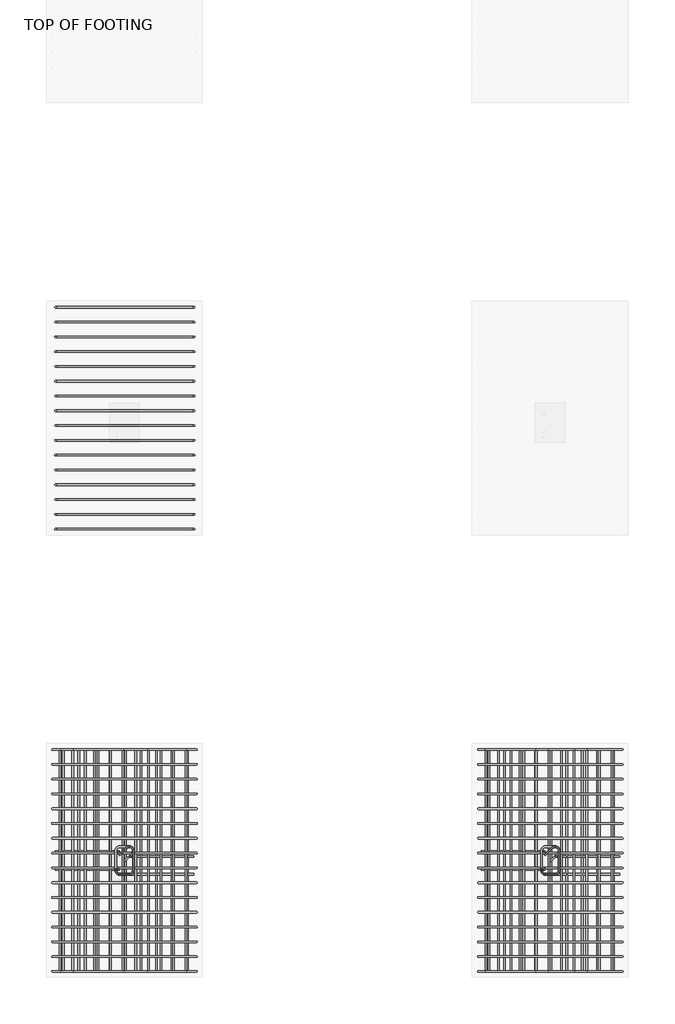
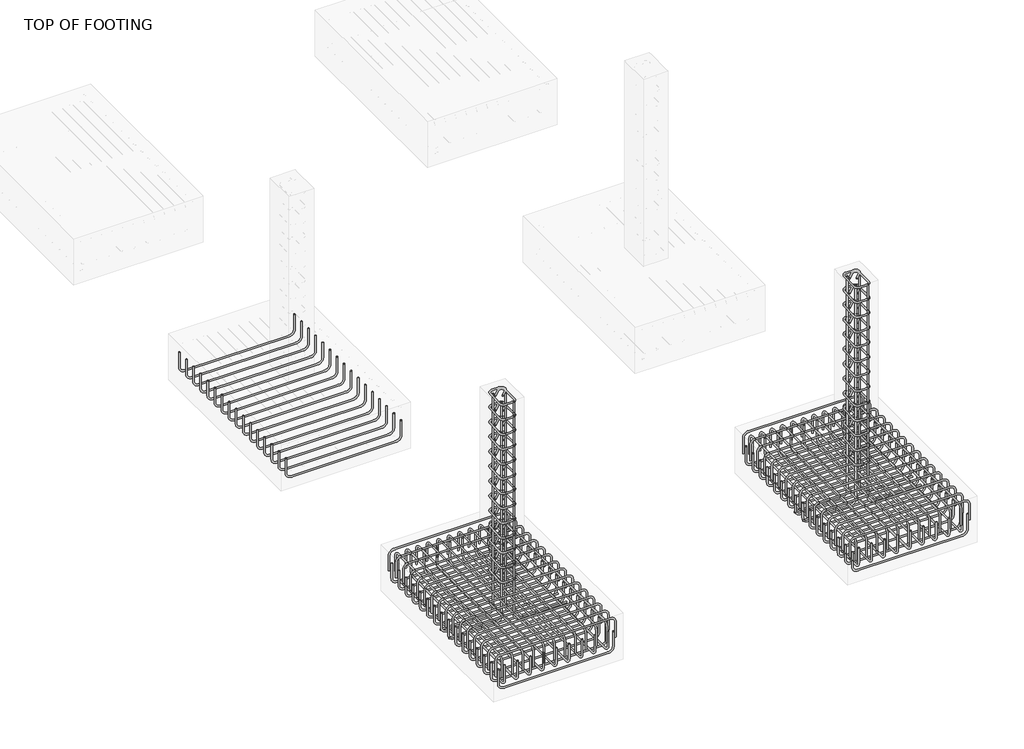
# One storey, part 2 of 8: 15 reinforcing bars.
"""IFC4 building model written with IfcOpenShell, lengths in millimetres."""

from ifc_helpers import new_model, si_unit, point, frame, origin, place, context, project, spatial, polyline, circle_curve, trimmed, segment, composite_curve, source, transform, mapped, element, save
from ifc_brep_helpers import swept_disk

model = new_model("IFC4")

# Units and contexts
model_context = context("Model", 3, world=origin())
ifc_project = project(units=[si_unit("LENGTHUNIT", "METRE", prefix="MILLI")], contexts=[model_context])

# Site, building, storey
site = spatial("IfcSite", under=ifc_project)
building = spatial("IfcBuilding", under=site)
storey = spatial("IfcBuildingStorey", under=building, Name="TOP OF FOOTING", Elevation=-1828.8)

# Reinforcing bars
placement = place(None, origin())
reinforcing_bar_shape = source(origin(), model_context, "Body", "SolidModel", [
    swept_disk(composite_curve([segment(polyline([(-4694.1573229, 6451.7662126, -2008.2544267), (-4694.1573229, 6451.7662126, -2155.5544267)]), True, "CONTINUOUS"), segment(trimmed(circle_curve(frame((-4740.5073229, 6451.7662126, -2155.5544267), z_axis=(0.0, 1.0, 0.0), x_axis=(46.350000000000364, 0.0, 0.0)), 46.35), [point((-4694.1573229, 6451.7662126, -2155.5544267))], [point((-4740.5073229, 6451.7662126, -2201.9044267))], True, "CARTESIAN"), True, "CONTINUOUS"), segment(polyline([(-4740.5073229, 6451.7662126, -2201.9044267), (-5711.5233592, 6451.7662126, -2201.9044267)]), True, "CONTINUOUS"), segment(trimmed(circle_curve(frame((-5711.5233592, 6451.7662126, -2155.5544267), z_axis=(0.0, 1.0, 0.0), x_axis=(0.0, 0.0, -46.34999999999991)), 46.35), [point((-5711.5233592, 6451.7662126, -2201.9044267))], [point((-5757.8733592, 6451.7662126, -2155.5544267))], True, "CARTESIAN"), True, "CONTINUOUS"), segment(polyline([(-5757.8733592, 6451.7662126, -2155.5544267), (-5757.8733592, 6451.7662126, -2008.2544267)]), True, "CONTINUOUS")], self_intersect=False), 6.35),
])
element("IfcReinforcingBar", 1, at=placement, inside=storey, context=model_context, shape_type="MappedRepresentation", body=[
    mapped(reinforcing_bar_shape, transform((0.0, 0.0, 0.0), x_axis=(1.0, 0.0, 0.0), y_axis=(0.0, 1.0, 0.0), z_axis=(0.0, 0.0, 1.0))),
    mapped(reinforcing_bar_shape, transform((0.0, -113.82, 0.0), x_axis=(1.0, 0.0, 0.0), y_axis=(0.0, 1.0, 0.0), z_axis=(0.0, 0.0, 1.0))),
    mapped(reinforcing_bar_shape, transform((0.0, -227.64, 0.0), x_axis=(1.0, 0.0, 0.0), y_axis=(0.0, 1.0, 0.0), z_axis=(0.0, 0.0, 1.0))),
    mapped(reinforcing_bar_shape, transform((0.0, -341.46, 0.0), x_axis=(1.0, 0.0, 0.0), y_axis=(0.0, 1.0, 0.0), z_axis=(0.0, 0.0, 1.0))),
    mapped(reinforcing_bar_shape, transform((0.0, -455.28, 0.0), x_axis=(1.0, 0.0, 0.0), y_axis=(0.0, 1.0, 0.0), z_axis=(0.0, 0.0, 1.0))),
    mapped(reinforcing_bar_shape, transform((0.0, -569.1, 0.0), x_axis=(1.0, 0.0, 0.0), y_axis=(0.0, 1.0, 0.0), z_axis=(0.0, 0.0, 1.0))),
    mapped(reinforcing_bar_shape, transform((0.0, -682.92, 0.0), x_axis=(1.0, 0.0, 0.0), y_axis=(0.0, 1.0, 0.0), z_axis=(0.0, 0.0, 1.0))),
    mapped(reinforcing_bar_shape, transform((0.0, -796.74, 0.0), x_axis=(1.0, 0.0, 0.0), y_axis=(0.0, 1.0, 0.0), z_axis=(0.0, 0.0, 1.0))),
    mapped(reinforcing_bar_shape, transform((0.0, -910.56, 0.0), x_axis=(1.0, 0.0, 0.0), y_axis=(0.0, 1.0, 0.0), z_axis=(0.0, 0.0, 1.0))),
    mapped(reinforcing_bar_shape, transform((0.0, -1024.38, 0.0), x_axis=(1.0, 0.0, 0.0), y_axis=(0.0, 1.0, 0.0), z_axis=(0.0, 0.0, 1.0))),
    mapped(reinforcing_bar_shape, transform((0.0, -1138.2, 0.0), x_axis=(1.0, 0.0, 0.0), y_axis=(0.0, 1.0, 0.0), z_axis=(0.0, 0.0, 1.0))),
    mapped(reinforcing_bar_shape, transform((0.0, -1252.02, 0.0), x_axis=(1.0, 0.0, 0.0), y_axis=(0.0, 1.0, 0.0), z_axis=(0.0, 0.0, 1.0))),
    mapped(reinforcing_bar_shape, transform((0.0, -1365.84, 0.0), x_axis=(1.0, 0.0, 0.0), y_axis=(0.0, 1.0, 0.0), z_axis=(0.0, 0.0, 1.0))),
    mapped(reinforcing_bar_shape, transform((0.0, -1479.66, 0.0), x_axis=(1.0, 0.0, 0.0), y_axis=(0.0, 1.0, 0.0), z_axis=(0.0, 0.0, 1.0))),
    mapped(reinforcing_bar_shape, transform((0.0, -1593.48, 0.0), x_axis=(1.0, 0.0, 0.0), y_axis=(0.0, 1.0, 0.0), z_axis=(0.0, 0.0, 1.0))),
    mapped(reinforcing_bar_shape, transform((0.0, -1707.3, 0.0), x_axis=(1.0, 0.0, 0.0), y_axis=(0.0, 1.0, 0.0), z_axis=(0.0, 0.0, 1.0))),
])
reinforcing_bar_2_shape = source(origin(), model_context, "Body", "SolidModel", [
    swept_disk(composite_curve([segment(polyline([(-5269.7182423, 2235.4007933, -46.35), (-5213.9746793, 2291.1443562, -46.35)]), True, "CONTINUOUS"), segment(trimmed(circle_curve(frame((-5191.8068817, 2268.9765586, -46.35), z_axis=(0.0, 0.0, -1.0), x_axis=(-22.167797600000085, 22.167797600000085, 0.0)), 31.35), [point((-5213.9746793, 2291.1443562, -46.35))], [point((-5160.4568817, 2268.9765586, -46.35))], True, "CARTESIAN"), True, "CONTINUOUS"), segment(polyline([(-5160.4568817, 2268.9765586, -46.35), (-5160.4568817, 2119.5765586, -46.35)]), True, "CONTINUOUS"), segment(trimmed(circle_curve(frame((-5191.8068817, 2119.5765586, -46.35), z_axis=(0.0, 0.0, -1.0), x_axis=(31.350000000000364, 0.0, 0.0)), 31.35), [point((-5160.4568817, 2119.5765586, -46.35))], [point((-5191.8068817, 2088.2265586, -46.35))], True, "CARTESIAN"), True, "CONTINUOUS"), segment(polyline([(-5191.8068817, 2088.2265586, -46.35), (-5265.0068817, 2088.2265586, -46.35)]), True, "CONTINUOUS"), segment(trimmed(circle_curve(frame((-5265.0068817, 2119.5205096, -44.4761991), z_axis=(0.0, 0.05977036468717588, -0.9982121535551258), x_axis=(0.0, -31.293951000000106, -1.873800899999999)), 31.35), [point((-5265.0068817, 2088.2265586, -46.35))], [point((-5296.3568817, 2119.5205096, -44.4761991))], True, "CARTESIAN"), True, "CONTINUOUS"), segment(polyline([(-5296.3568817, 2119.5205096, -44.4761991), (-5296.3568817, 2269.0326076, -35.5238009)]), True, "CONTINUOUS"), segment(trimmed(circle_curve(frame((-5265.0068817, 2269.0326076, -35.5238009), z_axis=(0.0, 0.05977036468717588, -0.9982121535551258), x_axis=(-31.349999999999454, 0.0, 0.0)), 31.35), [point((-5296.3568817, 2269.0326076, -35.5238009))], [point((-5265.0068817, 2300.3265586, -33.65))], True, "CARTESIAN"), True, "CONTINUOUS"), segment(polyline([(-5265.0068817, 2300.3265586, -33.65), (-5191.8068817, 2300.3265586, -33.65)]), True, "CONTINUOUS"), segment(trimmed(circle_curve(frame((-5191.8068817, 2268.9765586, -33.65), z_axis=(0.0, 0.0, -1.0), x_axis=(0.0, 31.350000000000364, 0.0)), 31.35), [point((-5191.8068817, 2300.3265586, -33.65))], [point((-5169.6390841, 2246.808761, -33.65))], True, "CARTESIAN"), True, "CONTINUOUS"), segment(polyline([(-5169.6390841, 2246.808761, -33.65), (-5225.3826471, 2191.0651981, -33.65)]), True, "CONTINUOUS")], self_intersect=False), 6.35),
])
element("IfcReinforcingBar", 2, at=placement, inside=storey, context=model_context, shape_type="MappedRepresentation", body=[
    mapped(reinforcing_bar_2_shape, transform((0.0, 0.0, 0.0), x_axis=(1.0, 0.0, 0.0), y_axis=(0.0, 1.0, 0.0), z_axis=(0.0, 0.0, 1.0))),
    mapped(reinforcing_bar_2_shape, transform((0.0, 0.0, -144.675), x_axis=(1.0, 0.0, 0.0), y_axis=(0.0, 1.0, 0.0), z_axis=(0.0, 0.0, 1.0))),
    mapped(reinforcing_bar_2_shape, transform((0.0, 0.0, -289.35), x_axis=(1.0, 0.0, 0.0), y_axis=(0.0, 1.0, 0.0), z_axis=(0.0, 0.0, 1.0))),
    mapped(reinforcing_bar_2_shape, transform((0.0, 0.0, -434.025), x_axis=(1.0, 0.0, 0.0), y_axis=(0.0, 1.0, 0.0), z_axis=(0.0, 0.0, 1.0))),
    mapped(reinforcing_bar_2_shape, transform((0.0, 0.0, -578.7), x_axis=(1.0, 0.0, 0.0), y_axis=(0.0, 1.0, 0.0), z_axis=(0.0, 0.0, 1.0))),
    mapped(reinforcing_bar_2_shape, transform((0.0, 0.0, -723.375), x_axis=(1.0, 0.0, 0.0), y_axis=(0.0, 1.0, 0.0), z_axis=(0.0, 0.0, 1.0))),
    mapped(reinforcing_bar_2_shape, transform((0.0, 0.0, -868.05), x_axis=(1.0, 0.0, 0.0), y_axis=(0.0, 1.0, 0.0), z_axis=(0.0, 0.0, 1.0))),
    mapped(reinforcing_bar_2_shape, transform((0.0, 0.0, -1012.725), x_axis=(1.0, 0.0, 0.0), y_axis=(0.0, 1.0, 0.0), z_axis=(0.0, 0.0, 1.0))),
    mapped(reinforcing_bar_2_shape, transform((0.0, 0.0, -1157.4), x_axis=(1.0, 0.0, 0.0), y_axis=(0.0, 1.0, 0.0), z_axis=(0.0, 0.0, 1.0))),
    mapped(reinforcing_bar_2_shape, transform((0.0, 0.0, -1302.075), x_axis=(1.0, 0.0, 0.0), y_axis=(0.0, 1.0, 0.0), z_axis=(0.0, 0.0, 1.0))),
    mapped(reinforcing_bar_2_shape, transform((0.0, 0.0, -1446.75), x_axis=(1.0, 0.0, 0.0), y_axis=(0.0, 1.0, 0.0), z_axis=(0.0, 0.0, 1.0))),
    mapped(reinforcing_bar_2_shape, transform((0.0, 0.0, -1591.425), x_axis=(1.0, 0.0, 0.0), y_axis=(0.0, 1.0, 0.0), z_axis=(0.0, 0.0, 1.0))),
    mapped(reinforcing_bar_2_shape, transform((0.0, 0.0, -1736.1), x_axis=(1.0, 0.0, 0.0), y_axis=(0.0, 1.0, 0.0), z_axis=(0.0, 0.0, 1.0))),
])
reinforcing_bar_3_shape = source(origin(), model_context, "Body", "SolidModel", [
    swept_disk(composite_curve([segment(polyline([(-4695.380398, 2088.2265586, -2177.1384798), (-5136.5372203, 2088.2265586, -2177.1384798)]), True, "CONTINUOUS"), segment(trimmed(circle_curve(frame((-5136.5372203, 2088.2265586, -2130.7884798), z_axis=(0.0, 1.0, 0.0), x_axis=(0.0, 0.0, -46.34999999999991)), 46.35), [point((-5136.5372203, 2088.2265586, -2177.1384798))], [point((-5182.8872203, 2088.2265586, -2130.7884798))], True, "CARTESIAN"), True, "CONTINUOUS"), segment(polyline([(-5182.8872203, 2088.2265586, -2130.7884798), (-5182.8872203, 2088.2265586, -40.0)]), True, "CONTINUOUS")], self_intersect=False), 6.35),
])
element("IfcReinforcingBar", 3, at=placement, inside=storey, context=model_context, shape_type="MappedRepresentation", body=[
    mapped(reinforcing_bar_3_shape, transform((0.0, 0.0, 0.0), x_axis=(1.0, 0.0, 0.0), y_axis=(0.0, 1.0, 0.0), z_axis=(0.0, 0.0, 1.0))),
    mapped(reinforcing_bar_3_shape, transform((0.0, 135.9, 0.0), x_axis=(1.0, 0.0, 0.0), y_axis=(0.0, 1.0, 0.0), z_axis=(0.0, 0.0, 1.0))),
])
reinforcing_bar_4_shape = source(origin(), model_context, "Body", "SolidModel", [
    swept_disk(composite_curve([segment(polyline([(-5761.4333654, 2126.3265586, -2177.1384798), (-5320.2765432, 2126.3265586, -2177.1384798)]), True, "CONTINUOUS"), segment(trimmed(circle_curve(frame((-5320.2765432, 2126.3265586, -2130.7884798), z_axis=(0.0, -1.0, 0.0), x_axis=(0.0, 0.0, -46.34999999999991)), 46.35), [point((-5320.2765432, 2126.3265586, -2177.1384798))], [point((-5273.9265432, 2126.3265586, -2130.7884798))], True, "CARTESIAN"), True, "CONTINUOUS"), segment(polyline([(-5273.9265432, 2126.3265586, -2130.7884798), (-5273.9265432, 2126.3265586, -40.0)]), True, "CONTINUOUS")], self_intersect=False), 6.35),
])
element("IfcReinforcingBar", 4, at=placement, inside=storey, context=model_context, shape_type="MappedRepresentation", body=[
    mapped(reinforcing_bar_4_shape, transform((0.0, 0.0, 0.0), x_axis=(1.0, 0.0, 0.0), y_axis=(0.0, 1.0, 0.0), z_axis=(0.0, 0.0, 1.0))),
    mapped(reinforcing_bar_4_shape, transform((0.0, 135.9, 0.0), x_axis=(1.0, 0.0, 0.0), y_axis=(0.0, 1.0, 0.0), z_axis=(0.0, 0.0, 1.0))),
])
reinforcing_bar_5_shape = source(origin(), model_context, "Body", "SolidModel", [
    swept_disk(composite_curve([segment(polyline([(-1993.1182423, 2235.4007933, -46.35), (-1937.3746793, 2291.1443562, -46.35)]), True, "CONTINUOUS"), segment(trimmed(circle_curve(frame((-1915.2068817, 2268.9765586, -46.35), z_axis=(0.0, 0.0, -1.0), x_axis=(-22.167797600000085, 22.167797600000085, 0.0)), 31.35), [point((-1937.3746793, 2291.1443562, -46.35))], [point((-1883.8568817, 2268.9765586, -46.35))], True, "CARTESIAN"), True, "CONTINUOUS"), segment(polyline([(-1883.8568817, 2268.9765586, -46.35), (-1883.8568817, 2119.5765586, -46.35)]), True, "CONTINUOUS"), segment(trimmed(circle_curve(frame((-1915.2068817, 2119.5765586, -46.35), z_axis=(0.0, 0.0, -1.0), x_axis=(31.34999999999991, 0.0, 0.0)), 31.35), [point((-1883.8568817, 2119.5765586, -46.35))], [point((-1915.2068817, 2088.2265586, -46.35))], True, "CARTESIAN"), True, "CONTINUOUS"), segment(polyline([(-1915.2068817, 2088.2265586, -46.35), (-1988.4068817, 2088.2265586, -46.35)]), True, "CONTINUOUS"), segment(trimmed(circle_curve(frame((-1988.4068817, 2119.5205096, -44.4761991), z_axis=(0.0, 0.05977036468717588, -0.9982121535551258), x_axis=(0.0, -31.293951000000106, -1.873800899999999)), 31.35), [point((-1988.4068817, 2088.2265586, -46.35))], [point((-2019.7568817, 2119.5205096, -44.4761991))], True, "CARTESIAN"), True, "CONTINUOUS"), segment(polyline([(-2019.7568817, 2119.5205096, -44.4761991), (-2019.7568817, 2269.0326076, -35.5238009)]), True, "CONTINUOUS"), segment(trimmed(circle_curve(frame((-1988.4068817, 2269.0326076, -35.5238009), z_axis=(0.0, 0.05977036468717588, -0.9982121535551258), x_axis=(-31.34999999999991, 0.0, 0.0)), 31.35), [point((-2019.7568817, 2269.0326076, -35.5238009))], [point((-1988.4068817, 2300.3265586, -33.65))], True, "CARTESIAN"), True, "CONTINUOUS"), segment(polyline([(-1988.4068817, 2300.3265586, -33.65), (-1915.2068817, 2300.3265586, -33.65)]), True, "CONTINUOUS"), segment(trimmed(circle_curve(frame((-1915.2068817, 2268.9765586, -33.65), z_axis=(0.0, 0.0, -1.0), x_axis=(0.0, 31.350000000000364, 0.0)), 31.35), [point((-1915.2068817, 2300.3265586, -33.65))], [point((-1893.0390841, 2246.808761, -33.65))], True, "CARTESIAN"), True, "CONTINUOUS"), segment(polyline([(-1893.0390841, 2246.808761, -33.65), (-1948.7826471, 2191.0651981, -33.65)]), True, "CONTINUOUS")], self_intersect=False), 6.35),
])
element("IfcReinforcingBar", 5, at=placement, inside=storey, context=model_context, shape_type="MappedRepresentation", body=[
    mapped(reinforcing_bar_5_shape, transform((0.0, 0.0, 0.0), x_axis=(1.0, 0.0, 0.0), y_axis=(0.0, 1.0, 0.0), z_axis=(0.0, 0.0, 1.0))),
    mapped(reinforcing_bar_5_shape, transform((0.0, 0.0, -144.675), x_axis=(1.0, 0.0, 0.0), y_axis=(0.0, 1.0, 0.0), z_axis=(0.0, 0.0, 1.0))),
    mapped(reinforcing_bar_5_shape, transform((0.0, 0.0, -289.35), x_axis=(1.0, 0.0, 0.0), y_axis=(0.0, 1.0, 0.0), z_axis=(0.0, 0.0, 1.0))),
    mapped(reinforcing_bar_5_shape, transform((0.0, 0.0, -434.025), x_axis=(1.0, 0.0, 0.0), y_axis=(0.0, 1.0, 0.0), z_axis=(0.0, 0.0, 1.0))),
    mapped(reinforcing_bar_5_shape, transform((0.0, 0.0, -578.7), x_axis=(1.0, 0.0, 0.0), y_axis=(0.0, 1.0, 0.0), z_axis=(0.0, 0.0, 1.0))),
    mapped(reinforcing_bar_5_shape, transform((0.0, 0.0, -723.375), x_axis=(1.0, 0.0, 0.0), y_axis=(0.0, 1.0, 0.0), z_axis=(0.0, 0.0, 1.0))),
    mapped(reinforcing_bar_5_shape, transform((0.0, 0.0, -868.05), x_axis=(1.0, 0.0, 0.0), y_axis=(0.0, 1.0, 0.0), z_axis=(0.0, 0.0, 1.0))),
    mapped(reinforcing_bar_5_shape, transform((0.0, 0.0, -1012.725), x_axis=(1.0, 0.0, 0.0), y_axis=(0.0, 1.0, 0.0), z_axis=(0.0, 0.0, 1.0))),
    mapped(reinforcing_bar_5_shape, transform((0.0, 0.0, -1157.4), x_axis=(1.0, 0.0, 0.0), y_axis=(0.0, 1.0, 0.0), z_axis=(0.0, 0.0, 1.0))),
    mapped(reinforcing_bar_5_shape, transform((0.0, 0.0, -1302.075), x_axis=(1.0, 0.0, 0.0), y_axis=(0.0, 1.0, 0.0), z_axis=(0.0, 0.0, 1.0))),
    mapped(reinforcing_bar_5_shape, transform((0.0, 0.0, -1446.75), x_axis=(1.0, 0.0, 0.0), y_axis=(0.0, 1.0, 0.0), z_axis=(0.0, 0.0, 1.0))),
    mapped(reinforcing_bar_5_shape, transform((0.0, 0.0, -1591.425), x_axis=(1.0, 0.0, 0.0), y_axis=(0.0, 1.0, 0.0), z_axis=(0.0, 0.0, 1.0))),
    mapped(reinforcing_bar_5_shape, transform((0.0, 0.0, -1736.1), x_axis=(1.0, 0.0, 0.0), y_axis=(0.0, 1.0, 0.0), z_axis=(0.0, 0.0, 1.0))),
])
reinforcing_bar_6_shape = source(origin(), model_context, "Body", "SolidModel", [
    swept_disk(composite_curve([segment(polyline([(-1418.780398, 2088.2265586, -2177.1384798), (-1859.9372203, 2088.2265586, -2177.1384798)]), True, "CONTINUOUS"), segment(trimmed(circle_curve(frame((-1859.9372203, 2088.2265586, -2130.7884798), z_axis=(0.0, 1.0, 0.0), x_axis=(0.0, 0.0, -46.34999999999991)), 46.35), [point((-1859.9372203, 2088.2265586, -2177.1384798))], [point((-1906.2872203, 2088.2265586, -2130.7884798))], True, "CARTESIAN"), True, "CONTINUOUS"), segment(polyline([(-1906.2872203, 2088.2265586, -2130.7884798), (-1906.2872203, 2088.2265586, -40.0)]), True, "CONTINUOUS")], self_intersect=False), 6.35),
])
element("IfcReinforcingBar", 6, at=placement, inside=storey, context=model_context, shape_type="MappedRepresentation", body=[
    mapped(reinforcing_bar_6_shape, transform((0.0, 0.0, 0.0), x_axis=(1.0, 0.0, 0.0), y_axis=(0.0, 1.0, 0.0), z_axis=(0.0, 0.0, 1.0))),
    mapped(reinforcing_bar_6_shape, transform((0.0, 135.9, 0.0), x_axis=(1.0, 0.0, 0.0), y_axis=(0.0, 1.0, 0.0), z_axis=(0.0, 0.0, 1.0))),
])
reinforcing_bar_7_shape = source(origin(), model_context, "Body", "SolidModel", [
    swept_disk(composite_curve([segment(polyline([(-2484.8333654, 2126.3265586, -2177.1384798), (-2043.6765432, 2126.3265586, -2177.1384798)]), True, "CONTINUOUS"), segment(trimmed(circle_curve(frame((-2043.6765432, 2126.3265586, -2130.7884798), z_axis=(0.0, -1.0, 0.0), x_axis=(0.0, 0.0, -46.34999999999991)), 46.35), [point((-2043.6765432, 2126.3265586, -2177.1384798))], [point((-1997.3265432, 2126.3265586, -2130.7884798))], True, "CARTESIAN"), True, "CONTINUOUS"), segment(polyline([(-1997.3265432, 2126.3265586, -2130.7884798), (-1997.3265432, 2126.3265586, -40.0)]), True, "CONTINUOUS")], self_intersect=False), 6.35),
])
element("IfcReinforcingBar", 7, at=placement, inside=storey, context=model_context, shape_type="MappedRepresentation", body=[
    mapped(reinforcing_bar_7_shape, transform((0.0, 0.0, 0.0), x_axis=(1.0, 0.0, 0.0), y_axis=(0.0, 1.0, 0.0), z_axis=(0.0, 0.0, 1.0))),
    mapped(reinforcing_bar_7_shape, transform((0.0, 135.9, 0.0), x_axis=(1.0, 0.0, 0.0), y_axis=(0.0, 1.0, 0.0), z_axis=(0.0, 0.0, 1.0))),
])
reinforcing_bar_8_shape = source(origin(), model_context, "Body", "SolidModel", [
    swept_disk(composite_curve([segment(polyline([(-4694.1573229, 3047.9265586, -2008.2544267), (-4694.1573229, 3047.9265586, -2155.5544267)]), True, "CONTINUOUS"), segment(trimmed(circle_curve(frame((-4740.5073229, 3047.9265586, -2155.5544267), z_axis=(0.0, 1.0, 0.0), x_axis=(46.350000000000364, 0.0, 0.0)), 46.35), [point((-4694.1573229, 3047.9265586, -2155.5544267))], [point((-4740.5073229, 3047.9265586, -2201.9044267))], True, "CARTESIAN"), True, "CONTINUOUS"), segment(polyline([(-4740.5073229, 3047.9265586, -2201.9044267), (-5711.5233592, 3047.9265586, -2201.9044267)]), True, "CONTINUOUS"), segment(trimmed(circle_curve(frame((-5711.5233592, 3047.9265586, -2155.5544267), z_axis=(0.0, 1.0, 0.0), x_axis=(0.0, 0.0, -46.34999999999991)), 46.35), [point((-5711.5233592, 3047.9265586, -2201.9044267))], [point((-5757.8733592, 3047.9265586, -2155.5544267))], True, "CARTESIAN"), True, "CONTINUOUS"), segment(polyline([(-5757.8733592, 3047.9265586, -2155.5544267), (-5757.8733592, 3047.9265586, -2008.2544267)]), True, "CONTINUOUS")], self_intersect=False), 6.35),
])
element("IfcReinforcingBar", 8, at=placement, inside=storey, context=model_context, shape_type="MappedRepresentation", body=[
    mapped(reinforcing_bar_8_shape, transform((0.0, 0.0, 0.0), x_axis=(1.0, 0.0, 0.0), y_axis=(0.0, 1.0, 0.0), z_axis=(0.0, 0.0, 1.0))),
    mapped(reinforcing_bar_8_shape, transform((0.0, -113.82, 0.0), x_axis=(1.0, 0.0, 0.0), y_axis=(0.0, 1.0, 0.0), z_axis=(0.0, 0.0, 1.0))),
    mapped(reinforcing_bar_8_shape, transform((0.0, -227.64, 0.0), x_axis=(1.0, 0.0, 0.0), y_axis=(0.0, 1.0, 0.0), z_axis=(0.0, 0.0, 1.0))),
    mapped(reinforcing_bar_8_shape, transform((0.0, -341.46, 0.0), x_axis=(1.0, 0.0, 0.0), y_axis=(0.0, 1.0, 0.0), z_axis=(0.0, 0.0, 1.0))),
    mapped(reinforcing_bar_8_shape, transform((0.0, -455.28, 0.0), x_axis=(1.0, 0.0, 0.0), y_axis=(0.0, 1.0, 0.0), z_axis=(0.0, 0.0, 1.0))),
    mapped(reinforcing_bar_8_shape, transform((0.0, -569.1, 0.0), x_axis=(1.0, 0.0, 0.0), y_axis=(0.0, 1.0, 0.0), z_axis=(0.0, 0.0, 1.0))),
    mapped(reinforcing_bar_8_shape, transform((0.0, -682.92, 0.0), x_axis=(1.0, 0.0, 0.0), y_axis=(0.0, 1.0, 0.0), z_axis=(0.0, 0.0, 1.0))),
    mapped(reinforcing_bar_8_shape, transform((0.0, -796.74, 0.0), x_axis=(1.0, 0.0, 0.0), y_axis=(0.0, 1.0, 0.0), z_axis=(0.0, 0.0, 1.0))),
    mapped(reinforcing_bar_8_shape, transform((0.0, -910.56, 0.0), x_axis=(1.0, 0.0, 0.0), y_axis=(0.0, 1.0, 0.0), z_axis=(0.0, 0.0, 1.0))),
    mapped(reinforcing_bar_8_shape, transform((0.0, -1024.38, 0.0), x_axis=(1.0, 0.0, 0.0), y_axis=(0.0, 1.0, 0.0), z_axis=(0.0, 0.0, 1.0))),
    mapped(reinforcing_bar_8_shape, transform((0.0, -1138.2, 0.0), x_axis=(1.0, 0.0, 0.0), y_axis=(0.0, 1.0, 0.0), z_axis=(0.0, 0.0, 1.0))),
    mapped(reinforcing_bar_8_shape, transform((0.0, -1252.02, 0.0), x_axis=(1.0, 0.0, 0.0), y_axis=(0.0, 1.0, 0.0), z_axis=(0.0, 0.0, 1.0))),
    mapped(reinforcing_bar_8_shape, transform((0.0, -1365.84, 0.0), x_axis=(1.0, 0.0, 0.0), y_axis=(0.0, 1.0, 0.0), z_axis=(0.0, 0.0, 1.0))),
    mapped(reinforcing_bar_8_shape, transform((0.0, -1479.66, 0.0), x_axis=(1.0, 0.0, 0.0), y_axis=(0.0, 1.0, 0.0), z_axis=(0.0, 0.0, 1.0))),
    mapped(reinforcing_bar_8_shape, transform((0.0, -1593.48, 0.0), x_axis=(1.0, 0.0, 0.0), y_axis=(0.0, 1.0, 0.0), z_axis=(0.0, 0.0, 1.0))),
    mapped(reinforcing_bar_8_shape, transform((0.0, -1707.3, 0.0), x_axis=(1.0, 0.0, 0.0), y_axis=(0.0, 1.0, 0.0), z_axis=(0.0, 0.0, 1.0))),
])
reinforcing_bar_9_shape = source(origin(), model_context, "Body", "SolidModel", [
    swept_disk(composite_curve([segment(polyline([(-5782.0568817, 3047.9265586, -2068.8), (-5782.0568817, 3047.9265586, -1921.5)]), True, "CONTINUOUS"), segment(trimmed(circle_curve(frame((-5735.7068817, 3047.9265586, -1921.5), z_axis=(0.0, 1.0, 0.0), x_axis=(-46.350000000000364, 0.0, 0.0)), 46.35), [point((-5782.0568817, 3047.9265586, -1921.5))], [point((-5735.7068817, 3047.9265586, -1875.15))], True, "CARTESIAN"), True, "CONTINUOUS"), segment(polyline([(-5735.7068817, 3047.9265586, -1875.15), (-4721.1068817, 3047.9265586, -1875.15)]), True, "CONTINUOUS"), segment(trimmed(circle_curve(frame((-4721.1068817, 3047.9265586, -1921.5), z_axis=(0.0, 1.0, 0.0), x_axis=(0.0, 0.0, 46.34999999999991)), 46.35), [point((-4721.1068817, 3047.9265586, -1875.15))], [point((-4674.7568817, 3047.9265586, -1921.5))], True, "CARTESIAN"), True, "CONTINUOUS"), segment(polyline([(-4674.7568817, 3047.9265586, -1921.5), (-4674.7568817, 3047.9265586, -2068.8)]), True, "CONTINUOUS")], self_intersect=False), 6.35),
])
element("IfcReinforcingBar", 9, at=placement, inside=storey, context=model_context, shape_type="MappedRepresentation", body=[
    mapped(reinforcing_bar_9_shape, transform((0.0, 0.0, 0.0), x_axis=(1.0, 0.0, 0.0), y_axis=(0.0, 1.0, 0.0), z_axis=(0.0, 0.0, 1.0))),
    mapped(reinforcing_bar_9_shape, transform((0.0, -113.82, 0.0), x_axis=(1.0, 0.0, 0.0), y_axis=(0.0, 1.0, 0.0), z_axis=(0.0, 0.0, 1.0))),
    mapped(reinforcing_bar_9_shape, transform((0.0, -227.64, 0.0), x_axis=(1.0, 0.0, 0.0), y_axis=(0.0, 1.0, 0.0), z_axis=(0.0, 0.0, 1.0))),
    mapped(reinforcing_bar_9_shape, transform((0.0, -341.46, 0.0), x_axis=(1.0, 0.0, 0.0), y_axis=(0.0, 1.0, 0.0), z_axis=(0.0, 0.0, 1.0))),
    mapped(reinforcing_bar_9_shape, transform((0.0, -455.28, 0.0), x_axis=(1.0, 0.0, 0.0), y_axis=(0.0, 1.0, 0.0), z_axis=(0.0, 0.0, 1.0))),
    mapped(reinforcing_bar_9_shape, transform((0.0, -569.1, 0.0), x_axis=(1.0, 0.0, 0.0), y_axis=(0.0, 1.0, 0.0), z_axis=(0.0, 0.0, 1.0))),
    mapped(reinforcing_bar_9_shape, transform((0.0, -682.92, 0.0), x_axis=(1.0, 0.0, 0.0), y_axis=(0.0, 1.0, 0.0), z_axis=(0.0, 0.0, 1.0))),
    mapped(reinforcing_bar_9_shape, transform((0.0, -796.74, 0.0), x_axis=(1.0, 0.0, 0.0), y_axis=(0.0, 1.0, 0.0), z_axis=(0.0, 0.0, 1.0))),
    mapped(reinforcing_bar_9_shape, transform((0.0, -910.56, 0.0), x_axis=(1.0, 0.0, 0.0), y_axis=(0.0, 1.0, 0.0), z_axis=(0.0, 0.0, 1.0))),
    mapped(reinforcing_bar_9_shape, transform((0.0, -1024.38, 0.0), x_axis=(1.0, 0.0, 0.0), y_axis=(0.0, 1.0, 0.0), z_axis=(0.0, 0.0, 1.0))),
    mapped(reinforcing_bar_9_shape, transform((0.0, -1138.2, 0.0), x_axis=(1.0, 0.0, 0.0), y_axis=(0.0, 1.0, 0.0), z_axis=(0.0, 0.0, 1.0))),
    mapped(reinforcing_bar_9_shape, transform((0.0, -1252.02, 0.0), x_axis=(1.0, 0.0, 0.0), y_axis=(0.0, 1.0, 0.0), z_axis=(0.0, 0.0, 1.0))),
    mapped(reinforcing_bar_9_shape, transform((0.0, -1365.84, 0.0), x_axis=(1.0, 0.0, 0.0), y_axis=(0.0, 1.0, 0.0), z_axis=(0.0, 0.0, 1.0))),
    mapped(reinforcing_bar_9_shape, transform((0.0, -1479.66, 0.0), x_axis=(1.0, 0.0, 0.0), y_axis=(0.0, 1.0, 0.0), z_axis=(0.0, 0.0, 1.0))),
    mapped(reinforcing_bar_9_shape, transform((0.0, -1593.48, 0.0), x_axis=(1.0, 0.0, 0.0), y_axis=(0.0, 1.0, 0.0), z_axis=(0.0, 0.0, 1.0))),
    mapped(reinforcing_bar_9_shape, transform((0.0, -1707.3, 0.0), x_axis=(1.0, 0.0, 0.0), y_axis=(0.0, 1.0, 0.0), z_axis=(0.0, 0.0, 1.0))),
])
reinforcing_bar_10_shape = source(origin(), model_context, "Body", "SolidModel", [
    swept_disk(composite_curve([segment(polyline([(-5699.8348303, 3047.9265586, -1986.9111268), (-5699.8348303, 3047.9265586, -2134.2111268)]), True, "CONTINUOUS"), segment(trimmed(circle_curve(frame((-5699.8348303, 3001.5765586, -2134.2111268), z_axis=(-1.0, 0.0, 0.0), x_axis=(0.0, 46.34999999999991, 0.0)), 46.35), [point((-5699.8348303, 3047.9265586, -2134.2111268))], [point((-5699.8348303, 3001.5765586, -2180.5611268))], True, "CARTESIAN"), True, "CONTINUOUS"), segment(polyline([(-5699.8348303, 3001.5765586, -2180.5611268), (-5699.8348303, 1386.9765586, -2180.5611268)]), True, "CONTINUOUS"), segment(trimmed(circle_curve(frame((-5699.8348303, 1386.9765586, -2134.2111268), z_axis=(-1.0, 0.0, 0.0), x_axis=(0.0, 0.0, -46.34999999999991)), 46.35), [point((-5699.8348303, 1386.9765586, -2180.5611268))], [point((-5699.8348303, 1340.6265586, -2134.2111268))], True, "CARTESIAN"), True, "CONTINUOUS"), segment(polyline([(-5699.8348303, 1340.6265586, -2134.2111268), (-5699.8348303, 1340.6265586, -1986.9111268)]), True, "CONTINUOUS")], self_intersect=False), 6.35),
])
element("IfcReinforcingBar", 10, at=placement, inside=storey, context=model_context, shape_type="MappedRepresentation", body=[
    mapped(reinforcing_bar_10_shape, transform((0.0, 0.0, 0.0), x_axis=(1.0, 0.0, 0.0), y_axis=(0.0, 1.0, 0.0), z_axis=(0.0, 0.0, 1.0))),
    mapped(reinforcing_bar_10_shape, transform((119.5564677, 0.0, 0.0), x_axis=(1.0, 0.0, 0.0), y_axis=(0.0, 1.0, 0.0), z_axis=(0.0, 0.0, 1.0))),
    mapped(reinforcing_bar_10_shape, transform((239.1129355, 0.0, 0.0), x_axis=(1.0, 0.0, 0.0), y_axis=(0.0, 1.0, 0.0), z_axis=(0.0, 0.0, 1.0))),
    mapped(reinforcing_bar_10_shape, transform((358.6694032, 0.0, 0.0), x_axis=(1.0, 0.0, 0.0), y_axis=(0.0, 1.0, 0.0), z_axis=(0.0, 0.0, 1.0))),
    mapped(reinforcing_bar_10_shape, transform((478.2258709, 0.0, 0.0), x_axis=(1.0, 0.0, 0.0), y_axis=(0.0, 1.0, 0.0), z_axis=(0.0, 0.0, 1.0))),
    mapped(reinforcing_bar_10_shape, transform((597.7823387, 0.0, 0.0), x_axis=(1.0, 0.0, 0.0), y_axis=(0.0, 1.0, 0.0), z_axis=(0.0, 0.0, 1.0))),
    mapped(reinforcing_bar_10_shape, transform((717.3388064, 0.0, 0.0), x_axis=(1.0, 0.0, 0.0), y_axis=(0.0, 1.0, 0.0), z_axis=(0.0, 0.0, 1.0))),
    mapped(reinforcing_bar_10_shape, transform((836.8952741, 0.0, 0.0), x_axis=(1.0, 0.0, 0.0), y_axis=(0.0, 1.0, 0.0), z_axis=(0.0, 0.0, 1.0))),
    mapped(reinforcing_bar_10_shape, transform((956.4517419, 0.0, 0.0), x_axis=(1.0, 0.0, 0.0), y_axis=(0.0, 1.0, 0.0), z_axis=(0.0, 0.0, 1.0))),
])
reinforcing_bar_11_shape = source(origin(), model_context, "Body", "SolidModel", [
    swept_disk(composite_curve([segment(polyline([(-4754.0668299, 3047.9265586, -2094.8977257), (-4754.0668299, 3047.9265586, -1947.5977257)]), True, "CONTINUOUS"), segment(trimmed(circle_curve(frame((-4754.0668299, 3001.5765586, -1947.5977257), z_axis=(1.0, 0.0, 0.0), x_axis=(0.0, 46.34999999999991, 0.0)), 46.35), [point((-4754.0668299, 3047.9265586, -1947.5977257))], [point((-4754.0668299, 3001.5765586, -1901.2477257))], True, "CARTESIAN"), True, "CONTINUOUS"), segment(polyline([(-4754.0668299, 3001.5765586, -1901.2477257), (-4754.0668299, 1386.9765586, -1901.2477257)]), True, "CONTINUOUS"), segment(trimmed(circle_curve(frame((-4754.0668299, 1386.9765586, -1947.5977257), z_axis=(1.0, 0.0, 0.0), x_axis=(0.0, 0.0, 46.34999999999991)), 46.35), [point((-4754.0668299, 1386.9765586, -1901.2477257))], [point((-4754.0668299, 1340.6265586, -1947.5977257))], True, "CARTESIAN"), True, "CONTINUOUS"), segment(polyline([(-4754.0668299, 1340.6265586, -1947.5977257), (-4754.0668299, 1340.6265586, -2094.8977257)]), True, "CONTINUOUS")], self_intersect=False), 6.35),
])
element("IfcReinforcingBar", 11, at=placement, inside=storey, context=model_context, shape_type="MappedRepresentation", body=[
    mapped(reinforcing_bar_11_shape, transform((0.0, 0.0, 0.0), x_axis=(1.0, 0.0, 0.0), y_axis=(0.0, 1.0, 0.0), z_axis=(0.0, 0.0, 1.0))),
    mapped(reinforcing_bar_11_shape, transform((-97.0050815, 0.0, 0.0), x_axis=(1.0, 0.0, 0.0), y_axis=(0.0, 1.0, 0.0), z_axis=(0.0, 0.0, 1.0))),
    mapped(reinforcing_bar_11_shape, transform((-194.0101631, 0.0, 0.0), x_axis=(1.0, 0.0, 0.0), y_axis=(0.0, 1.0, 0.0), z_axis=(0.0, 0.0, 1.0))),
    mapped(reinforcing_bar_11_shape, transform((-291.0152446, 0.0, 0.0), x_axis=(1.0, 0.0, 0.0), y_axis=(0.0, 1.0, 0.0), z_axis=(0.0, 0.0, 1.0))),
    mapped(reinforcing_bar_11_shape, transform((-388.0203261, 0.0, 0.0), x_axis=(1.0, 0.0, 0.0), y_axis=(0.0, 1.0, 0.0), z_axis=(0.0, 0.0, 1.0))),
    mapped(reinforcing_bar_11_shape, transform((-485.0254076, 0.0, 0.0), x_axis=(1.0, 0.0, 0.0), y_axis=(0.0, 1.0, 0.0), z_axis=(0.0, 0.0, 1.0))),
    mapped(reinforcing_bar_11_shape, transform((-582.0304892, 0.0, 0.0), x_axis=(1.0, 0.0, 0.0), y_axis=(0.0, 1.0, 0.0), z_axis=(0.0, 0.0, 1.0))),
    mapped(reinforcing_bar_11_shape, transform((-679.0355707, 0.0, 0.0), x_axis=(1.0, 0.0, 0.0), y_axis=(0.0, 1.0, 0.0), z_axis=(0.0, 0.0, 1.0))),
    mapped(reinforcing_bar_11_shape, transform((-776.0406522, 0.0, 0.0), x_axis=(1.0, 0.0, 0.0), y_axis=(0.0, 1.0, 0.0), z_axis=(0.0, 0.0, 1.0))),
    mapped(reinforcing_bar_11_shape, transform((-873.0457338, 0.0, 0.0), x_axis=(1.0, 0.0, 0.0), y_axis=(0.0, 1.0, 0.0), z_axis=(0.0, 0.0, 1.0))),
    mapped(reinforcing_bar_11_shape, transform((-970.0508153, 0.0, 0.0), x_axis=(1.0, 0.0, 0.0), y_axis=(0.0, 1.0, 0.0), z_axis=(0.0, 0.0, 1.0))),
])
reinforcing_bar_12_shape = source(origin(), model_context, "Body", "SolidModel", [
    swept_disk(composite_curve([segment(polyline([(-1417.5573229, 3047.9265586, -2008.2544267), (-1417.5573229, 3047.9265586, -2155.5544267)]), True, "CONTINUOUS"), segment(trimmed(circle_curve(frame((-1463.9073229, 3047.9265586, -2155.5544267), z_axis=(0.0, 1.0, 0.0), x_axis=(46.350000000000136, 0.0, 0.0)), 46.35), [point((-1417.5573229, 3047.9265586, -2155.5544267))], [point((-1463.9073229, 3047.9265586, -2201.9044267))], True, "CARTESIAN"), True, "CONTINUOUS"), segment(polyline([(-1463.9073229, 3047.9265586, -2201.9044267), (-2434.9233592, 3047.9265586, -2201.9044267)]), True, "CONTINUOUS"), segment(trimmed(circle_curve(frame((-2434.9233592, 3047.9265586, -2155.5544267), z_axis=(0.0, 1.0, 0.0), x_axis=(0.0, 0.0, -46.34999999999991)), 46.35), [point((-2434.9233592, 3047.9265586, -2201.9044267))], [point((-2481.2733592, 3047.9265586, -2155.5544267))], True, "CARTESIAN"), True, "CONTINUOUS"), segment(polyline([(-2481.2733592, 3047.9265586, -2155.5544267), (-2481.2733592, 3047.9265586, -2008.2544267)]), True, "CONTINUOUS")], self_intersect=False), 6.35),
])
element("IfcReinforcingBar", 12, at=placement, inside=storey, context=model_context, shape_type="MappedRepresentation", body=[
    mapped(reinforcing_bar_12_shape, transform((0.0, 0.0, 0.0), x_axis=(1.0, 0.0, 0.0), y_axis=(0.0, 1.0, 0.0), z_axis=(0.0, 0.0, 1.0))),
    mapped(reinforcing_bar_12_shape, transform((0.0, -113.82, 0.0), x_axis=(1.0, 0.0, 0.0), y_axis=(0.0, 1.0, 0.0), z_axis=(0.0, 0.0, 1.0))),
    mapped(reinforcing_bar_12_shape, transform((0.0, -227.64, 0.0), x_axis=(1.0, 0.0, 0.0), y_axis=(0.0, 1.0, 0.0), z_axis=(0.0, 0.0, 1.0))),
    mapped(reinforcing_bar_12_shape, transform((0.0, -341.46, 0.0), x_axis=(1.0, 0.0, 0.0), y_axis=(0.0, 1.0, 0.0), z_axis=(0.0, 0.0, 1.0))),
    mapped(reinforcing_bar_12_shape, transform((0.0, -455.28, 0.0), x_axis=(1.0, 0.0, 0.0), y_axis=(0.0, 1.0, 0.0), z_axis=(0.0, 0.0, 1.0))),
    mapped(reinforcing_bar_12_shape, transform((0.0, -569.1, 0.0), x_axis=(1.0, 0.0, 0.0), y_axis=(0.0, 1.0, 0.0), z_axis=(0.0, 0.0, 1.0))),
    mapped(reinforcing_bar_12_shape, transform((0.0, -682.92, 0.0), x_axis=(1.0, 0.0, 0.0), y_axis=(0.0, 1.0, 0.0), z_axis=(0.0, 0.0, 1.0))),
    mapped(reinforcing_bar_12_shape, transform((0.0, -796.74, 0.0), x_axis=(1.0, 0.0, 0.0), y_axis=(0.0, 1.0, 0.0), z_axis=(0.0, 0.0, 1.0))),
    mapped(reinforcing_bar_12_shape, transform((0.0, -910.56, 0.0), x_axis=(1.0, 0.0, 0.0), y_axis=(0.0, 1.0, 0.0), z_axis=(0.0, 0.0, 1.0))),
    mapped(reinforcing_bar_12_shape, transform((0.0, -1024.38, 0.0), x_axis=(1.0, 0.0, 0.0), y_axis=(0.0, 1.0, 0.0), z_axis=(0.0, 0.0, 1.0))),
    mapped(reinforcing_bar_12_shape, transform((0.0, -1138.2, 0.0), x_axis=(1.0, 0.0, 0.0), y_axis=(0.0, 1.0, 0.0), z_axis=(0.0, 0.0, 1.0))),
    mapped(reinforcing_bar_12_shape, transform((0.0, -1252.02, 0.0), x_axis=(1.0, 0.0, 0.0), y_axis=(0.0, 1.0, 0.0), z_axis=(0.0, 0.0, 1.0))),
    mapped(reinforcing_bar_12_shape, transform((0.0, -1365.84, 0.0), x_axis=(1.0, 0.0, 0.0), y_axis=(0.0, 1.0, 0.0), z_axis=(0.0, 0.0, 1.0))),
    mapped(reinforcing_bar_12_shape, transform((0.0, -1479.66, 0.0), x_axis=(1.0, 0.0, 0.0), y_axis=(0.0, 1.0, 0.0), z_axis=(0.0, 0.0, 1.0))),
    mapped(reinforcing_bar_12_shape, transform((0.0, -1593.48, 0.0), x_axis=(1.0, 0.0, 0.0), y_axis=(0.0, 1.0, 0.0), z_axis=(0.0, 0.0, 1.0))),
    mapped(reinforcing_bar_12_shape, transform((0.0, -1707.3, 0.0), x_axis=(1.0, 0.0, 0.0), y_axis=(0.0, 1.0, 0.0), z_axis=(0.0, 0.0, 1.0))),
])
reinforcing_bar_13_shape = source(origin(), model_context, "Body", "SolidModel", [
    swept_disk(composite_curve([segment(polyline([(-2505.4568817, 3047.9265586, -2068.8), (-2505.4568817, 3047.9265586, -1921.5)]), True, "CONTINUOUS"), segment(trimmed(circle_curve(frame((-2459.1068817, 3047.9265586, -1921.5), z_axis=(0.0, 1.0, 0.0), x_axis=(-46.34999999999991, 0.0, 0.0)), 46.35), [point((-2505.4568817, 3047.9265586, -1921.5))], [point((-2459.1068817, 3047.9265586, -1875.15))], True, "CARTESIAN"), True, "CONTINUOUS"), segment(polyline([(-2459.1068817, 3047.9265586, -1875.15), (-1444.5068817, 3047.9265586, -1875.15)]), True, "CONTINUOUS"), segment(trimmed(circle_curve(frame((-1444.5068817, 3047.9265586, -1921.5), z_axis=(0.0, 1.0, 0.0), x_axis=(0.0, 0.0, 46.34999999999991)), 46.35), [point((-1444.5068817, 3047.9265586, -1875.15))], [point((-1398.1568817, 3047.9265586, -1921.5))], True, "CARTESIAN"), True, "CONTINUOUS"), segment(polyline([(-1398.1568817, 3047.9265586, -1921.5), (-1398.1568817, 3047.9265586, -2068.8)]), True, "CONTINUOUS")], self_intersect=False), 6.35),
])
element("IfcReinforcingBar", 13, at=placement, inside=storey, context=model_context, shape_type="MappedRepresentation", body=[
    mapped(reinforcing_bar_13_shape, transform((0.0, 0.0, 0.0), x_axis=(1.0, 0.0, 0.0), y_axis=(0.0, 1.0, 0.0), z_axis=(0.0, 0.0, 1.0))),
    mapped(reinforcing_bar_13_shape, transform((0.0, -113.82, 0.0), x_axis=(1.0, 0.0, 0.0), y_axis=(0.0, 1.0, 0.0), z_axis=(0.0, 0.0, 1.0))),
    mapped(reinforcing_bar_13_shape, transform((0.0, -227.64, 0.0), x_axis=(1.0, 0.0, 0.0), y_axis=(0.0, 1.0, 0.0), z_axis=(0.0, 0.0, 1.0))),
    mapped(reinforcing_bar_13_shape, transform((0.0, -341.46, 0.0), x_axis=(1.0, 0.0, 0.0), y_axis=(0.0, 1.0, 0.0), z_axis=(0.0, 0.0, 1.0))),
    mapped(reinforcing_bar_13_shape, transform((0.0, -455.28, 0.0), x_axis=(1.0, 0.0, 0.0), y_axis=(0.0, 1.0, 0.0), z_axis=(0.0, 0.0, 1.0))),
    mapped(reinforcing_bar_13_shape, transform((0.0, -569.1, 0.0), x_axis=(1.0, 0.0, 0.0), y_axis=(0.0, 1.0, 0.0), z_axis=(0.0, 0.0, 1.0))),
    mapped(reinforcing_bar_13_shape, transform((0.0, -682.92, 0.0), x_axis=(1.0, 0.0, 0.0), y_axis=(0.0, 1.0, 0.0), z_axis=(0.0, 0.0, 1.0))),
    mapped(reinforcing_bar_13_shape, transform((0.0, -796.74, 0.0), x_axis=(1.0, 0.0, 0.0), y_axis=(0.0, 1.0, 0.0), z_axis=(0.0, 0.0, 1.0))),
    mapped(reinforcing_bar_13_shape, transform((0.0, -910.56, 0.0), x_axis=(1.0, 0.0, 0.0), y_axis=(0.0, 1.0, 0.0), z_axis=(0.0, 0.0, 1.0))),
    mapped(reinforcing_bar_13_shape, transform((0.0, -1024.38, 0.0), x_axis=(1.0, 0.0, 0.0), y_axis=(0.0, 1.0, 0.0), z_axis=(0.0, 0.0, 1.0))),
    mapped(reinforcing_bar_13_shape, transform((0.0, -1138.2, 0.0), x_axis=(1.0, 0.0, 0.0), y_axis=(0.0, 1.0, 0.0), z_axis=(0.0, 0.0, 1.0))),
    mapped(reinforcing_bar_13_shape, transform((0.0, -1252.02, 0.0), x_axis=(1.0, 0.0, 0.0), y_axis=(0.0, 1.0, 0.0), z_axis=(0.0, 0.0, 1.0))),
    mapped(reinforcing_bar_13_shape, transform((0.0, -1365.84, 0.0), x_axis=(1.0, 0.0, 0.0), y_axis=(0.0, 1.0, 0.0), z_axis=(0.0, 0.0, 1.0))),
    mapped(reinforcing_bar_13_shape, transform((0.0, -1479.66, 0.0), x_axis=(1.0, 0.0, 0.0), y_axis=(0.0, 1.0, 0.0), z_axis=(0.0, 0.0, 1.0))),
    mapped(reinforcing_bar_13_shape, transform((0.0, -1593.48, 0.0), x_axis=(1.0, 0.0, 0.0), y_axis=(0.0, 1.0, 0.0), z_axis=(0.0, 0.0, 1.0))),
    mapped(reinforcing_bar_13_shape, transform((0.0, -1707.3, 0.0), x_axis=(1.0, 0.0, 0.0), y_axis=(0.0, 1.0, 0.0), z_axis=(0.0, 0.0, 1.0))),
])
reinforcing_bar_14_shape = source(origin(), model_context, "Body", "SolidModel", [
    swept_disk(composite_curve([segment(polyline([(-2423.2348303, 3047.9265586, -1986.9111268), (-2423.2348303, 3047.9265586, -2134.2111268)]), True, "CONTINUOUS"), segment(trimmed(circle_curve(frame((-2423.2348303, 3001.5765586, -2134.2111268), z_axis=(-1.0, 0.0, 0.0), x_axis=(0.0, 46.34999999999991, 0.0)), 46.35), [point((-2423.2348303, 3047.9265586, -2134.2111268))], [point((-2423.2348303, 3001.5765586, -2180.5611268))], True, "CARTESIAN"), True, "CONTINUOUS"), segment(polyline([(-2423.2348303, 3001.5765586, -2180.5611268), (-2423.2348303, 1386.9765586, -2180.5611268)]), True, "CONTINUOUS"), segment(trimmed(circle_curve(frame((-2423.2348303, 1386.9765586, -2134.2111268), z_axis=(-1.0, 0.0, 0.0), x_axis=(0.0, 0.0, -46.34999999999991)), 46.35), [point((-2423.2348303, 1386.9765586, -2180.5611268))], [point((-2423.2348303, 1340.6265586, -2134.2111268))], True, "CARTESIAN"), True, "CONTINUOUS"), segment(polyline([(-2423.2348303, 1340.6265586, -2134.2111268), (-2423.2348303, 1340.6265586, -1986.9111268)]), True, "CONTINUOUS")], self_intersect=False), 6.35),
])
element("IfcReinforcingBar", 14, at=placement, inside=storey, context=model_context, shape_type="MappedRepresentation", body=[
    mapped(reinforcing_bar_14_shape, transform((0.0, 0.0, 0.0), x_axis=(1.0, 0.0, 0.0), y_axis=(0.0, 1.0, 0.0), z_axis=(0.0, 0.0, 1.0))),
    mapped(reinforcing_bar_14_shape, transform((119.5564677, 0.0, 0.0), x_axis=(1.0, 0.0, 0.0), y_axis=(0.0, 1.0, 0.0), z_axis=(0.0, 0.0, 1.0))),
    mapped(reinforcing_bar_14_shape, transform((239.1129355, 0.0, 0.0), x_axis=(1.0, 0.0, 0.0), y_axis=(0.0, 1.0, 0.0), z_axis=(0.0, 0.0, 1.0))),
    mapped(reinforcing_bar_14_shape, transform((358.6694032, 0.0, 0.0), x_axis=(1.0, 0.0, 0.0), y_axis=(0.0, 1.0, 0.0), z_axis=(0.0, 0.0, 1.0))),
    mapped(reinforcing_bar_14_shape, transform((478.2258709, 0.0, 0.0), x_axis=(1.0, 0.0, 0.0), y_axis=(0.0, 1.0, 0.0), z_axis=(0.0, 0.0, 1.0))),
    mapped(reinforcing_bar_14_shape, transform((597.7823387, 0.0, 0.0), x_axis=(1.0, 0.0, 0.0), y_axis=(0.0, 1.0, 0.0), z_axis=(0.0, 0.0, 1.0))),
    mapped(reinforcing_bar_14_shape, transform((717.3388064, 0.0, 0.0), x_axis=(1.0, 0.0, 0.0), y_axis=(0.0, 1.0, 0.0), z_axis=(0.0, 0.0, 1.0))),
    mapped(reinforcing_bar_14_shape, transform((836.8952741, 0.0, 0.0), x_axis=(1.0, 0.0, 0.0), y_axis=(0.0, 1.0, 0.0), z_axis=(0.0, 0.0, 1.0))),
    mapped(reinforcing_bar_14_shape, transform((956.4517419, 0.0, 0.0), x_axis=(1.0, 0.0, 0.0), y_axis=(0.0, 1.0, 0.0), z_axis=(0.0, 0.0, 1.0))),
])
reinforcing_bar_15_shape = source(origin(), model_context, "Body", "SolidModel", [
    swept_disk(composite_curve([segment(polyline([(-1477.4668299, 3047.9265586, -2094.8977257), (-1477.4668299, 3047.9265586, -1947.5977257)]), True, "CONTINUOUS"), segment(trimmed(circle_curve(frame((-1477.4668299, 3001.5765586, -1947.5977257), z_axis=(1.0, 0.0, 0.0), x_axis=(0.0, 46.34999999999991, 0.0)), 46.35), [point((-1477.4668299, 3047.9265586, -1947.5977257))], [point((-1477.4668299, 3001.5765586, -1901.2477257))], True, "CARTESIAN"), True, "CONTINUOUS"), segment(polyline([(-1477.4668299, 3001.5765586, -1901.2477257), (-1477.4668299, 1386.9765586, -1901.2477257)]), True, "CONTINUOUS"), segment(trimmed(circle_curve(frame((-1477.4668299, 1386.9765586, -1947.5977257), z_axis=(1.0, 0.0, 0.0), x_axis=(0.0, 0.0, 46.34999999999991)), 46.35), [point((-1477.4668299, 1386.9765586, -1901.2477257))], [point((-1477.4668299, 1340.6265586, -1947.5977257))], True, "CARTESIAN"), True, "CONTINUOUS"), segment(polyline([(-1477.4668299, 1340.6265586, -1947.5977257), (-1477.4668299, 1340.6265586, -2094.8977257)]), True, "CONTINUOUS")], self_intersect=False), 6.35),
])
element("IfcReinforcingBar", 15, at=placement, inside=storey, context=model_context, shape_type="MappedRepresentation", body=[
    mapped(reinforcing_bar_15_shape, transform((0.0, 0.0, 0.0), x_axis=(1.0, 0.0, 0.0), y_axis=(0.0, 1.0, 0.0), z_axis=(0.0, 0.0, 1.0))),
    mapped(reinforcing_bar_15_shape, transform((-97.0050815, 0.0, 0.0), x_axis=(1.0, 0.0, 0.0), y_axis=(0.0, 1.0, 0.0), z_axis=(0.0, 0.0, 1.0))),
    mapped(reinforcing_bar_15_shape, transform((-194.0101631, 0.0, 0.0), x_axis=(1.0, 0.0, 0.0), y_axis=(0.0, 1.0, 0.0), z_axis=(0.0, 0.0, 1.0))),
    mapped(reinforcing_bar_15_shape, transform((-291.0152446, 0.0, 0.0), x_axis=(1.0, 0.0, 0.0), y_axis=(0.0, 1.0, 0.0), z_axis=(0.0, 0.0, 1.0))),
    mapped(reinforcing_bar_15_shape, transform((-388.0203261, 0.0, 0.0), x_axis=(1.0, 0.0, 0.0), y_axis=(0.0, 1.0, 0.0), z_axis=(0.0, 0.0, 1.0))),
    mapped(reinforcing_bar_15_shape, transform((-485.0254076, 0.0, 0.0), x_axis=(1.0, 0.0, 0.0), y_axis=(0.0, 1.0, 0.0), z_axis=(0.0, 0.0, 1.0))),
    mapped(reinforcing_bar_15_shape, transform((-582.0304892, 0.0, 0.0), x_axis=(1.0, 0.0, 0.0), y_axis=(0.0, 1.0, 0.0), z_axis=(0.0, 0.0, 1.0))),
    mapped(reinforcing_bar_15_shape, transform((-679.0355707, 0.0, 0.0), x_axis=(1.0, 0.0, 0.0), y_axis=(0.0, 1.0, 0.0), z_axis=(0.0, 0.0, 1.0))),
    mapped(reinforcing_bar_15_shape, transform((-776.0406522, 0.0, 0.0), x_axis=(1.0, 0.0, 0.0), y_axis=(0.0, 1.0, 0.0), z_axis=(0.0, 0.0, 1.0))),
    mapped(reinforcing_bar_15_shape, transform((-873.0457338, 0.0, 0.0), x_axis=(1.0, 0.0, 0.0), y_axis=(0.0, 1.0, 0.0), z_axis=(0.0, 0.0, 1.0))),
    mapped(reinforcing_bar_15_shape, transform((-970.0508153, 0.0, 0.0), x_axis=(1.0, 0.0, 0.0), y_axis=(0.0, 1.0, 0.0), z_axis=(0.0, 0.0, 1.0))),
])

save(model, "model.ifc")

# Revit data of these elements
# Elements 1, 2, 3, 4, 5, 6, 7, 8, 9, 10, 11, 12, 13, 14, 15 (IfcReinforcingBar)
#   Phase Created = New Construction
